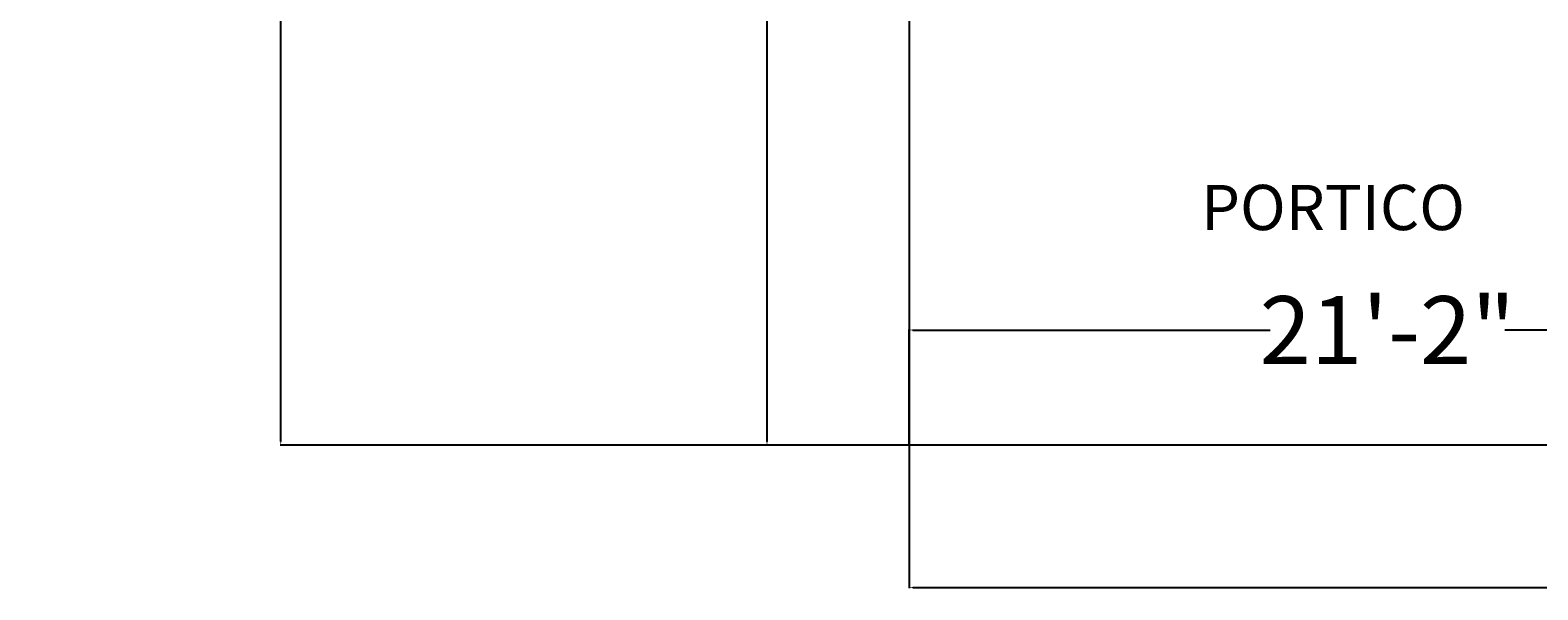
# Model space of a CAD drawing. Units: inches. Extents: x -304 to 580, y 363 to 1149.
# Tile 1 of 11: x -304 to 96, y 364 to 512. Entities that reach past the tile are written whole.
import ezdxf

# ---------------------------------------------------------------- set-up
doc = ezdxf.new("R2010")
doc.units = ezdxf.units.IN
doc.header["$MEASUREMENT"] = 0
for name, color, linetype, lineweight in [('A-ANNO-DIMS', 2, 'Continuous', 13), ('A-AREA-IDEN', 7, 'Continuous', 25), ('A-FLOR-OTLN', 2, 'Continuous', 25)]:
    doc.layers.add(name, color=color, linetype=linetype, lineweight=lineweight)
doc.styles.get("Standard").update_dxf_attribs({"font": 'arial.ttf'})
doc.dimstyles.get("Standard").update_dxf_attribs({"dimtxt": 1, "dimasz": 1, "dimexe": 0.18, "dimexo": 0.0625, "dimgap": 0.09, "dimtad": 0, "dimtih": 1, "dimtoh": 1, "dimdec": 0, "dimzin": 0, "dimdsep": 46, "dimlunit": 3, "dimtxsty": 'Standard', "dimcen": 0.09, "dimadec": 0, "dimazin": 0, "dimtfac": 1, "dimtdec": 0, "dimtofl": 0, "dimtmove": 0, "dimatfit": 3, "dimfxl": 1, "dimtolj": 1, "dimtzin": 0, "dimarcsym": 0})

# ---------------------------------------------------------------- blocks, each defined once
blk = doc.blocks.new('*D1')
at = {"layer": 'A-ANNO-DIMS', "color": 0, "lineweight": -2, "transparency": 16777216}
for p, q in [((-22.63, 1004.95), (-237.62, 1004.95)), ((-237.44, 1003.95), (-237.44, 721.93)), ((-237.44, 402.95), (-237.44, 684.96)), ((-22.63, 401.95), (-237.62, 401.95))]:
    blk.add_line(p, q, dxfattribs=at)
at = {"layer": 'A-ANNO-DIMS', "color": 0, "transparency": 16777216}
for points in [[(-237.61, 1003.95), (-237.28, 1003.95), (-237.44, 1004.95)], [(-237.61, 402.95), (-237.28, 402.95), (-237.44, 401.95)]]:
    blk.add_solid(points, dxfattribs=at)
at = {"layer": 'Defpoints', "color": 0, "transparency": 16777216}
for p in [(-22.57, 1004.95), (-237.44, 401.95), (-22.57, 401.95)]:
    blk.add_point(p, dxfattribs=at)
at = {"layer": 'A-ANNO-DIMS', "color": 0, "transparency": 16777216, "insert": (-237.44, 703.45), "char_height": 1, "attachment_point": 5}
blk.add_mtext('\\A1;{\\H36x;50\'-3"}', dxfattribs=at)
blk = doc.blocks.new('*D22')
at = {"layer": 'A-ANNO-DIMS', "color": 0, "lineweight": -2, "transparency": 16777216}
for p, q in [((-70.57, 402.01), (-70.57, 432.73)), ((-69.57, 432.55), (25.27, 432.55)), ((182.43, 432.55), (87.59, 432.55)), ((183.43, 402.01), (183.43, 432.73))]:
    blk.add_line(p, q, dxfattribs=at)
at = {"layer": 'A-ANNO-DIMS', "color": 0, "transparency": 16777216}
for points in [[(-69.57, 432.72), (-69.57, 432.38), (-70.57, 432.55)], [(182.43, 432.72), (182.43, 432.38), (183.43, 432.55)]]:
    blk.add_solid(points, dxfattribs=at)
at = {"layer": 'Defpoints', "color": 0, "transparency": 16777216}
for p in [(183.43, 432.55), (-70.57, 401.95), (183.43, 401.95)]:
    blk.add_point(p, dxfattribs=at)
at = {"layer": 'A-ANNO-DIMS', "color": 0, "transparency": 16777216, "insert": (56.43, 432.55), "char_height": 1, "attachment_point": 5}
blk.add_mtext('\\A1;{\\H18x;21\'-2"}', dxfattribs=at)
blk = doc.blocks.new('*D29')
at = {"layer": 'A-ANNO-DIMS', "color": 0, "lineweight": -2, "transparency": 16777216}
for p, q in [((316.43, 410.88), (316.43, 364.02)), ((-70.57, 401.88), (-70.57, 364.02)), ((-69.57, 364.2), (121.12, 364.2)), ((315.43, 364.2), (124.74, 364.2))]:
    blk.add_line(p, q, dxfattribs=at)
at = {"layer": 'A-ANNO-DIMS', "color": 0, "transparency": 16777216}
for points in [[(-69.57, 364.36), (-69.57, 364.03), (-70.57, 364.2)], [(315.43, 364.36), (315.43, 364.03), (316.43, 364.2)]]:
    blk.add_solid(points, dxfattribs=at)
at = {"layer": 'Defpoints', "color": 0, "transparency": 16777216}
for p in [(316.43, 410.95), (-70.57, 401.95), (316.43, 364.2)]:
    blk.add_point(p, dxfattribs=at)
at = {"layer": 'A-ANNO-DIMS', "color": 0, "transparency": 16777216, "insert": (122.93, 364.2), "char_height": 1, "attachment_point": 5}
blk.add_mtext('\\A1;32\'-3"', dxfattribs=at)
blk = doc.blocks.new('*D30')
at = {"layer": 'A-ANNO-DIMS', "color": 0, "lineweight": -2, "transparency": 16777216}
for p, q in [((-70.63, 721.98), (-108.5, 721.98)), ((-108.32, 720.98), (-108.32, 562.56)), ((-108.32, 402.95), (-108.32, 561.36)), ((-70.63, 401.95), (-108.5, 401.95))]:
    blk.add_line(p, q, dxfattribs=at)
at = {"layer": 'A-ANNO-DIMS', "color": 0, "transparency": 16777216}
for points in [[(-108.49, 720.98), (-108.15, 720.98), (-108.32, 721.98)], [(-108.49, 402.95), (-108.15, 402.95), (-108.32, 401.95)]]:
    blk.add_solid(points, dxfattribs=at)
at = {"layer": 'Defpoints', "color": 0, "transparency": 16777216}
for p in [(-108.32, 721.98), (-70.57, 721.98), (-70.57, 401.95)]:
    blk.add_point(p, dxfattribs=at)
at = {"layer": 'A-ANNO-DIMS', "color": 0, "transparency": 16777216, "insert": (-108.32, 561.96), "char_height": 1, "attachment_point": 5}
blk.add_mtext('\\A1;26\'-8"', dxfattribs=at)

msp = doc.modelspace()

# ---------------------------------------------------------------- linework, layer by layer
at = {"layer": 'A-FLOR-OTLN'}
for p in [(-70.57, 721.98), (183.43, 401.95)]:
    msp.add_line(p, (-70.57, 401.95), dxfattribs=at)

# ---------------------------------------------------------------- texts
at = {"layer": 'A-AREA-IDEN', "insert": (6.92, 471.1), "char_height": 12, "attachment_point": 1}
msp.add_mtext_dynamic_manual_height_columns('PORTICO', width=39.4169, gutter_width=1, heights=[0], dxfattribs=at)

# ---------------------------------------------------------------- dimensions: what is measured, and where the dimension line sits
at = {"layer": 'A-ANNO-DIMS'}
dim = msp.add_linear_dim(base=(-237.44, 401.95), p1=(-22.57, 1004.95), p2=(-22.57, 401.95), angle=90, text='{\\H36x;<>}', dimstyle='Standard', override={"dimclrd": 0, "dimclre": 0, "dimclrt": 0}, dxfattribs=at)
dim.commit()
dim.dimension.update_dxf_attribs({"geometry": '*D1', "text_midpoint": (-237.44, 703.45)})
dim = msp.add_linear_dim(base=(-108.32, 721.98), p1=(-70.57, 401.95), p2=(-70.57, 721.98), angle=90, dimstyle='Standard', override={"dimdec": 1, "dimlfac": 1, "dimrnd": 0, "dimzin": 1, "dimdsep": 46, "dimlunit": 4, "dimfrac": 2}, dxfattribs=at)
dim.commit()
dim.dimension.update_dxf_attribs({"geometry": '*D30', "text_midpoint": (-108.32, 561.96)})
dim = msp.add_linear_dim(base=(183.43, 432.55), p1=(-70.57, 401.95), p2=(183.43, 401.95), text='{\\H18x;<>}', dimstyle='Standard', override={"dimclrd": 0, "dimclre": 0, "dimclrt": 0}, dxfattribs=at)
dim.commit()
dim.dimension.update_dxf_attribs({"geometry": '*D22', "text_midpoint": (56.43, 432.55)})
dim = msp.add_linear_dim(base=(316.43, 364.2), p1=(-70.57, 401.95), p2=(316.43, 410.95), dimstyle='Standard', override={"dimdec": 1, "dimlfac": 1, "dimrnd": 0, "dimzin": 1, "dimdsep": 46, "dimlunit": 4, "dimfrac": 2}, dxfattribs=at)
dim.commit()
dim.dimension.update_dxf_attribs({"geometry": '*D29', "text_midpoint": (122.93, 364.2)})

doc.saveas('drawing.dxf')
